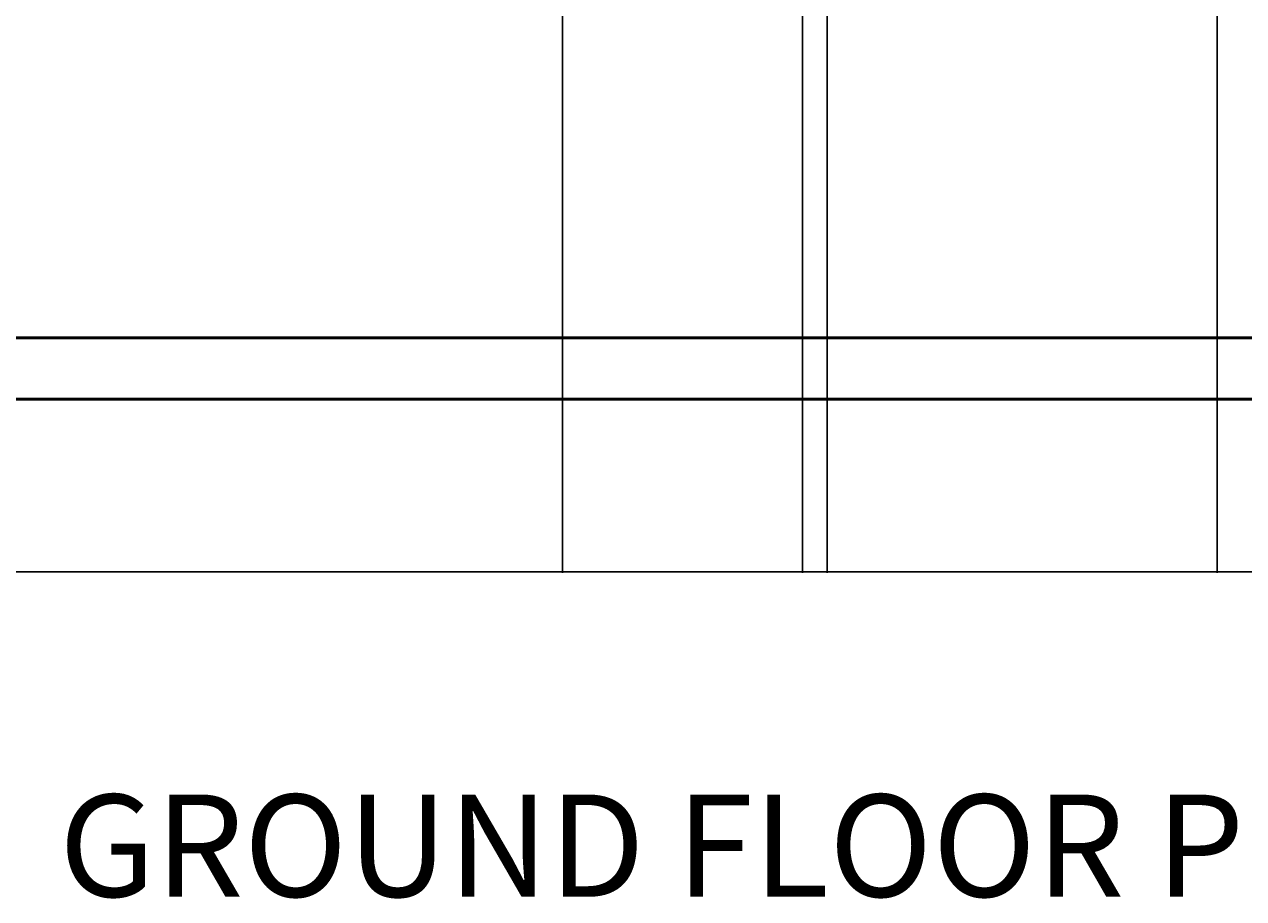
# Model space of a CAD drawing. Units: inches. Extents: x -1517 to -668, y -425 to 52.
# Tile 2 of 13: x -1365 to -1186, y -425 to -296. Entities that reach past the tile are written whole.
import ezdxf

# ---------------------------------------------------------------- set-up
doc = ezdxf.new("R2010")
doc.units = ezdxf.units.IN
doc.header["$MEASUREMENT"] = 0
for name, color, linetype, lineweight in [('A-ANNO-DIMS', 2, 'Continuous', 18), ('A-ANNO-TEXT', 7, 'Continuous', 18), ('walls', 240, 'Continuous', 50)]:
    doc.layers.add(name, color=color, linetype=linetype, lineweight=lineweight)
doc.styles.get("Standard").update_dxf_attribs({"font": 'arial.ttf'})
doc.dimstyles.get("Standard").update_dxf_attribs({"dimtxt": 0.18, "dimasz": 0.18, "dimexe": 0.18, "dimexo": 0.0625, "dimgap": 0.09, "dimtad": 0, "dimtih": 1, "dimtoh": 1, "dimdec": 4, "dimzin": 0, "dimdsep": 46, "dimlunit": 4, "dimtxsty": 'Standard', "dimcen": 0.09, "dimadec": 0, "dimazin": 0, "dimtfac": 1, "dimtdec": 4, "dimtofl": 0, "dimtmove": 0, "dimatfit": 3, "dimfxl": 1, "dimtolj": 1, "dimtzin": 0, "dimarcsym": 0})

# ---------------------------------------------------------------- blocks, each defined once
blk = doc.blocks.new('*D44')
at = {"layer": 'A-ANNO-DIMS', "color": 0, "lineweight": -2, "transparency": 16777216}
for p, q in [((-1491.5, -351.43), (-1491.5, -376.85)), ((-1005.5, -351.43), (-1005.5, -376.85)), ((-1491.32, -376.67), (-1248.8, -376.67)), ((-1005.68, -376.67), (-1248.21, -376.67))]:
    blk.add_line(p, q, dxfattribs=at)
at = {"layer": 'A-ANNO-DIMS', "color": 0, "transparency": 16777216}
for points in [[(-1491.32, -376.64), (-1491.32, -376.7), (-1491.5, -376.67)], [(-1005.68, -376.64), (-1005.68, -376.7), (-1005.5, -376.67)]]:
    blk.add_solid(points, dxfattribs=at)
at = {"layer": 'Defpoints', "color": 0, "transparency": 16777216}
for p in [(-1491.5, -351.37), (-1005.5, -351.37), (-1005.5, -376.67)]:
    blk.add_point(p, dxfattribs=at)
at = {"layer": 'A-ANNO-DIMS', "color": 0, "transparency": 16777216, "insert": (-1248.5, -376.67), "char_height": 0.18, "attachment_point": 5}
blk.add_mtext('\\A1;486', dxfattribs=at)
blk = doc.blocks.new('*D48')
at = {"layer": 'A-ANNO-DIMS', "color": 0, "lineweight": -2, "transparency": 16777216}
for p, q in [((-1285.9, -102.43), (-1285.9, -376.85)), ((-1189.9, -102.43), (-1189.9, -376.85)), ((-1285.72, -376.67), (-1238.12, -376.67)), ((-1190.08, -376.67), (-1237.68, -376.67))]:
    blk.add_line(p, q, dxfattribs=at)
at = {"layer": 'A-ANNO-DIMS', "color": 0, "transparency": 16777216}
for points in [[(-1285.72, -376.64), (-1285.72, -376.7), (-1285.9, -376.67)], [(-1190.08, -376.64), (-1190.08, -376.7), (-1189.9, -376.67)]]:
    blk.add_solid(points, dxfattribs=at)
at = {"layer": 'Defpoints', "color": 0, "transparency": 16777216}
for p in [(-1285.9, -102.37), (-1189.9, -102.37), (-1189.9, -376.67)]:
    blk.add_point(p, dxfattribs=at)
at = {"layer": 'A-ANNO-DIMS', "color": 0, "transparency": 16777216, "insert": (-1237.9, -376.67), "char_height": 0.18, "attachment_point": 5}
blk.add_mtext('\\A1;96', dxfattribs=at)
blk = doc.blocks.new('*D71')
at = {"layer": 'A-ANNO-DIMS', "color": 0, "lineweight": -2, "transparency": 16777216}
for p, q in [((-1250.69, -158.03), (-1250.69, -376.85)), ((-1247.1, -158.03), (-1247.1, -376.85)), ((-1250.51, -376.67), (-1249.29, -376.67)), ((-1247.28, -376.67), (-1248.5, -376.67))]:
    blk.add_line(p, q, dxfattribs=at)
at = {"layer": 'A-ANNO-DIMS', "color": 0, "transparency": 16777216}
for points in [[(-1250.51, -376.64), (-1250.51, -376.7), (-1250.69, -376.67)], [(-1247.28, -376.64), (-1247.28, -376.7), (-1247.1, -376.67)]]:
    blk.add_solid(points, dxfattribs=at)
at = {"layer": 'Defpoints', "color": 0, "transparency": 16777216}
for p in [(-1250.69, -157.97), (-1247.1, -157.97), (-1247.1, -376.67)]:
    blk.add_point(p, dxfattribs=at)
at = {"layer": 'A-ANNO-DIMS', "color": 0, "transparency": 16777216, "insert": (-1248.9, -376.67), "char_height": 0.18, "attachment_point": 5}
blk.add_mtext('\\A1;3.583', dxfattribs=at)

msp = doc.modelspace()

# ---------------------------------------------------------------- linework, layer by layer
at = {"layer": 'walls'}
for p, q in [((-1482.5037, -342.37), (-1014.5037, -342.37)), ((-1491.5037, -351.37), (-1005.5037, -351.37))]:
    msp.add_line(p, q, dxfattribs=at)

# ---------------------------------------------------------------- texts
at = {"layer": 'A-ANNO-TEXT', "insert": (-1359.7191, -409.3504), "char_height": 15, "attachment_point": 1}
msp.add_mtext_dynamic_manual_height_columns('{\\fArial|b1|i0|c0|p34;GROUND FLOOR PLAN}', width=581.299229, gutter_width=1, heights=[0], dxfattribs=at)

# ---------------------------------------------------------------- dimensions: what is measured, and where the dimension line sits
at = {"layer": 'A-ANNO-DIMS'}
for base, p1, p2, override, picture, middle in [((-1189.9037, -376.67), (-1285.9037, -102.37), (-1189.9037, -102.37), {"dimdec": 0, "dimlfac": 1, "dimrnd": 0, "dimzin": 0, "dimdsep": 46, "dimlunit": 2}, '*D48', (-1237.9037, -376.67)), ((-1247.1037, -376.67), (-1250.687, -157.97), (-1247.1037, -157.97), {"dimdec": 3, "dimlfac": 1, "dimrnd": 0, "dimzin": 0, "dimdsep": 46, "dimlunit": 2}, '*D71', (-1248.8953, -376.67)), ((-1005.5037, -376.67), (-1491.5037, -351.37), (-1005.5037, -351.37), {"dimdec": 0, "dimlfac": 1, "dimrnd": 0, "dimzin": 0, "dimdsep": 46, "dimlunit": 2}, '*D44', (-1248.5037, -376.67))]:
    dim = msp.add_linear_dim(base=base, p1=p1, p2=p2, dimstyle='Standard', override=override, dxfattribs=at)
    dim.commit()
    dim.dimension.update_dxf_attribs({"geometry": picture, "text_midpoint": middle})

doc.saveas('drawing.dxf')
